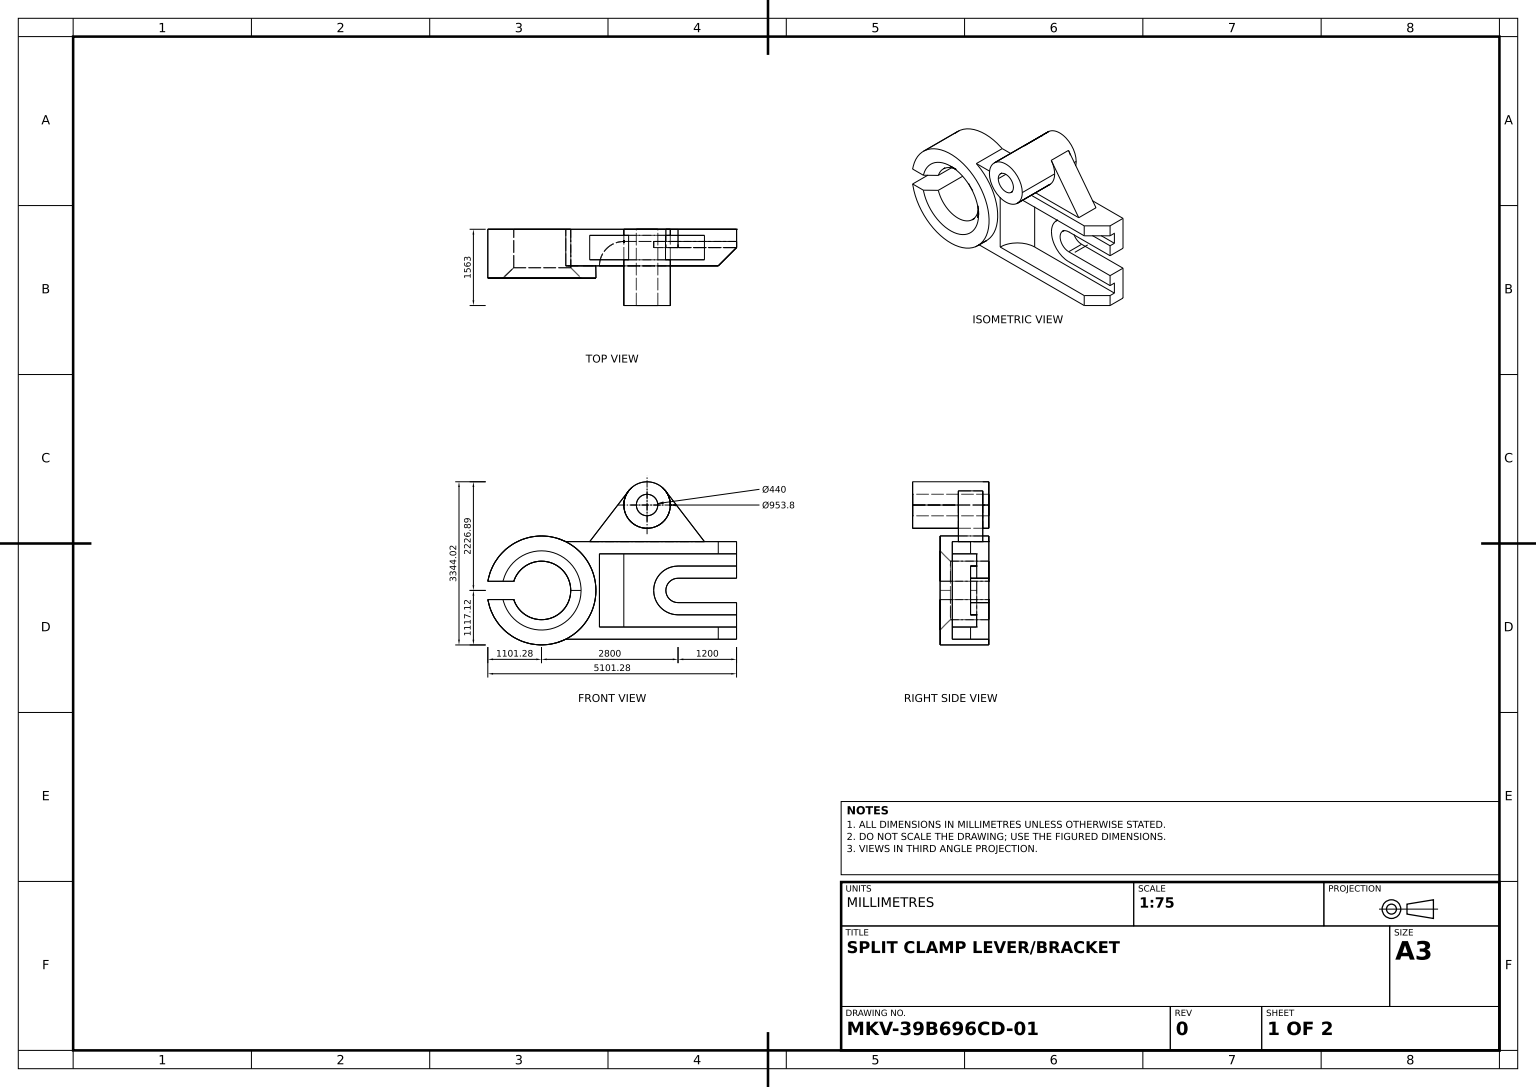
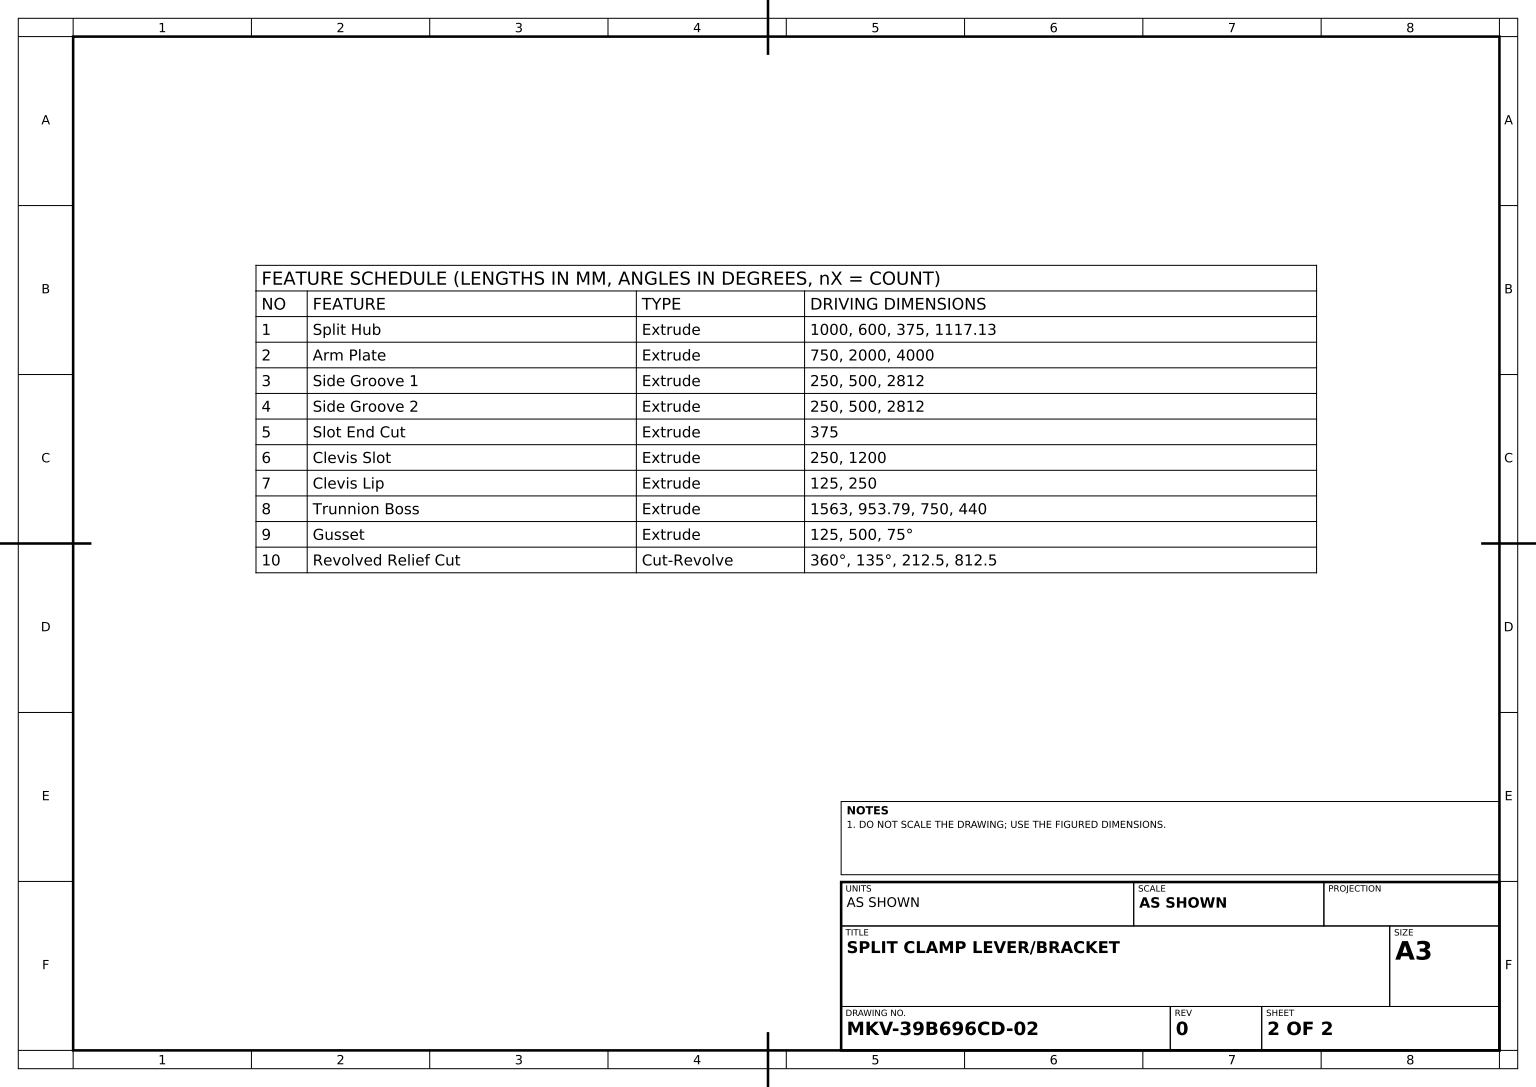
from build123d import *

# Parameters (mm, degrees)
SPLIT_HUB_DEPTH          = 1000
ARM_PLATE_DEPTH          = 750
SIDE_GROOVE_1_DEPTH      = 750
SIDE_START               = -750
SIDE_GROOVE_2_DEPTH      = 750
SLOT_END_CUT_DEPTH       = 4635.893681294
CLEVIS_SLOT_DEPTH        = 4221.246371588
CLEVIS_START             = 125
CLEVIS_LIP_DEPTH         = 125
TRUNNION_BOSS_SKETCH_R   = 476.895
TRUNNION_BOSS_SKETCH_R_2 = 220
TRUNNION_BOSS_DEPTH      = 1563
GUSSET_DEPTH             = 500


with BuildPart() as part:
    # Hub Profile Sketch → Split Hub (new body)
    with BuildSketch(Plane.XY):
        with BuildLine():
            Line((-1101.282519111, 187.5), (-569.950655759, 187.5))
            ThreePointArc((-569.950655759, 187.5), (600, 0), (-569.950655759, -187.5))
            Line((-569.950655759, -187.5), (-1101.282519111, -187.5))
            ThreePointArc((-1101.282519111, -187.5), (1117.13, 0), (-1101.282519111, 187.5))
        make_face()
    extrude(amount=SPLIT_HUB_DEPTH)

    # Arm Plate Sketch → Arm Plate (add)
    with BuildSketch(Plane.XY):
        with BuildLine():
            Line((497.975337642, 1000), (4000, 1000))
            Line((4000, 1000), (4000, -1000))
            Line((4000, -1000), (497.975337642, -1000))
            ThreePointArc((497.975337642, -1000), (1117.13, 0), (497.975337642, 1000))
        make_face()
    extrude(amount=ARM_PLATE_DEPTH)

    # Side Groove Sketch → Side Groove 1 (cut)
    with BuildSketch(Plane(origin=(0, 0, 0), x_dir=(1, 0, 0), z_dir=(0, 1, 0))):
        with BuildLine():
            Line((4000, -250), (1688, -250))
            ThreePointArc((1688, -250), (1334.446609407, -396.446609407), (1188, -750))
            Line((1188, -750), (4000, -750))
            Line((4000, -750), (4000, -250))
        make_face()
    extrude(amount=SIDE_GROOVE_1_DEPTH, mode=Mode.SUBTRACT)

    # Sketch3_2 → Side Groove 2 (cut)
    with BuildSketch(Plane(origin=(0, 0, 0), x_dir=(1, 0, 0), z_dir=(0, 1, 0)).offset(SIDE_START)):
        with BuildLine():
            Line((4000, -250), (1688, -250))
            ThreePointArc((1688, -250), (1334.446609407, -396.446609407), (1188, -750))
            Line((1188, -750), (4000, -750))
            Line((4000, -750), (4000, -250))
        make_face()
    extrude(amount=SIDE_GROOVE_2_DEPTH, mode=Mode.SUBTRACT)

    # Slot End Sketch → Slot End Cut (cut, through all)
    with BuildSketch(Plane(origin=(0, 1000, 0), x_dir=(1, 0, 0), z_dir=(0, 1, 0))):
        Polygon((4000, -375), (3625, -750), (4000, -750), align=None)
    extrude(amount=-SLOT_END_CUT_DEPTH, mode=Mode.SUBTRACT)

    # Clevis Slot Sketch → Clevis Slot (cut, through all)
    with BuildSketch(Plane.XY.offset(250)):
        with BuildLine():
            Line((2800, 250), (4000, 250))
            Line((4000, 250), (4000, -250))
            Line((4000, -250), (2800, -250))
            ThreePointArc((2800, -250), (2550, 0), (2800, 250))
        make_face()
    extrude(amount=-CLEVIS_SLOT_DEPTH, mode=Mode.SUBTRACT)

    # Clevis Lip Sketch → Clevis Lip (add)
    with BuildSketch(Plane.XY.offset(250).offset(CLEVIS_START)):
        with BuildLine():
            Line((2800, -250), (4000, -250))
            Line((4000, -250), (4000, -500))
            Line((4000, -500), (2800, -500))
            ThreePointArc((2800, -500), (2300, 0), (2800, 500))
            Line((2800, 500), (4000, 500))
            Line((4000, 500), (4000, 250))
            Line((4000, 250), (2800, 250))
            ThreePointArc((2800, 250), (2550, 0), (2800, -250))
        make_face()
    extrude(amount=-CLEVIS_LIP_DEPTH)



with BuildPart() as body_2:
    # Trunnion Boss Sketch → Trunnion Boss (new body)
    with BuildSketch(Plane(origin=(0, 0, 0), x_dir=(-1, 0, 0), z_dir=(0, 0, -1))):
        with Locations((-2164.895, 1750)):
            Circle(TRUNNION_BOSS_SKETCH_R)
        with Locations((-2164.895, 1750)):
            Circle(TRUNNION_BOSS_SKETCH_R_2, mode=Mode.SUBTRACT)
    extrude(amount=-TRUNNION_BOSS_DEPTH)


with BuildPart() as part_1:
    add(part.part)

    add(body_2.part)  # Gusset merges body 2
    # Gusset Sketch → Gusset (add)
    with BuildSketch(Plane.XY.offset(125)):
        with BuildLine():
            Line((2543.241241218, 2040.315281687), (3341.503232864, 1000))
            Line((3341.503232864, 1000), (988.286767136, 1000))
            Line((988.286767136, 1000), (1786.548758782, 2040.315281687))
            ThreePointArc((1786.548758782, 2040.315281687), (2164.895, 1273.105), (2543.241241218, 2040.315281687))
        make_face()
    extrude(amount=GUSSET_DEPTH)

    # Revolved Cut Sketch → Revolved Relief Cut (revolve, cut)
    with BuildSketch(Plane(origin=(0, 0, 0), x_dir=(0, 0, -1), z_dir=(1, 0, 0))):
        Polygon((0, 600), (-787.5, 600), (-1000, 812.5), (-1000, 0), (0, 0), align=None)
    revolve(axis=Axis((0, 0, 0), (0, 0, 1)), mode=Mode.SUBTRACT)


solid = part_1.part
